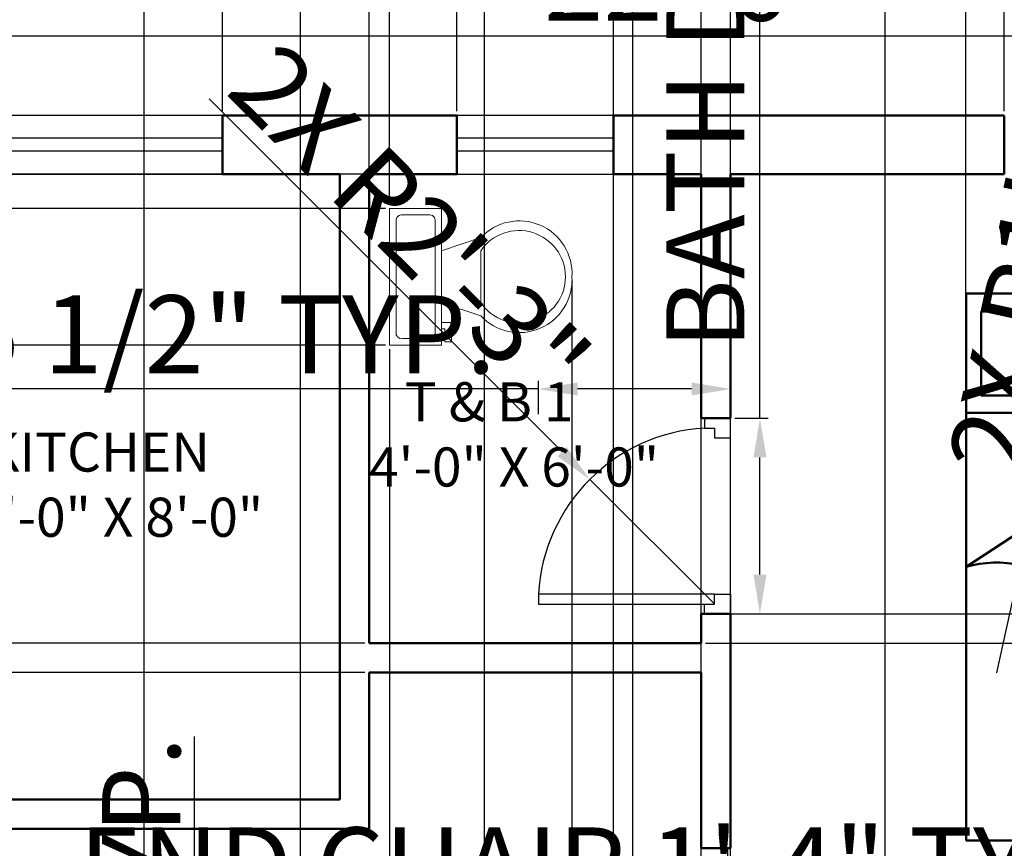
# Model space of a CAD drawing. Units: inches. Extents: x 1086 to 1501, y 383 to 973.
# Tile 5 of 7: x 1165 to 1316, y 723 to 850. Entities that reach past the tile are written whole.
import ezdxf

# ---------------------------------------------------------------- set-up
doc = ezdxf.new("R2010")
doc.units = ezdxf.units.IN
for name, color, linetype, lineweight in [('A-ANNO-DIMS', 2, 'Continuous', 18), ('A-AREA-IDEN', 7, 'Continuous', 25), ('A-FLOR-FIXT', 9, 'Continuous', 18), ('door', 10, 'Continuous', 25), ('furniture', 255, 'Continuous', 18), ('ventilator', 151, 'Continuous', 25), ('wall', 7, 'Continuous', 50), ('window', 81, 'Continuous', 25)]:
    doc.layers.add(name, color=color, linetype=linetype, lineweight=lineweight)
doc.styles.get("Standard").update_dxf_attribs({"font": 'arial.ttf'})
doc.dimstyles.new('ISO-25', dxfattribs={"dimtxt": 12, "dimasz": 6, "dimexe": 1.25, "dimexo": 0.625, "dimtad": 1, "dimdec": 1, "dimlunit": 3, "dimtxsty": 'Standard', "dimcen": 2.5, "dimadec": 0, "dimazin": 0, "dimtfac": 1, "dimtdec": 1, "dimtmove": 0, "dimatfit": 3, "dimfxl": 1, "dimarcsym": 0})

# ---------------------------------------------------------------- blocks, each defined once
blk = doc.blocks.new('w1')
at = {"layer": 'window'}
for p, q in [((1475.33, 845.32), (1475.33, 809.32)), ((1477.33, 845.32), (1477.33, 809.32))]:
    blk.add_line(p, q, dxfattribs=at)
blk.add_lwpolyline([(1471.83, 809.32), (1480.83, 809.32), (1480.83, 845.32), (1471.83, 845.32)], close=True, dxfattribs=at)
blk = doc.blocks.new('v')
at = {"layer": 'ventilator'}
for p, q in [((1539.56, 920.22), (1539.56, 896.22)), ((1541.56, 920.22), (1541.56, 896.22))]:
    blk.add_line(p, q, dxfattribs=at)
blk.add_lwpolyline([(1536.06, 896.22), (1545.06, 896.22), (1545.06, 920.22), (1536.06, 920.22)], close=True, dxfattribs=at)
blk = doc.blocks.new('d2')
at = {"layer": 'door'}
blk.add_line((1603.89, 600.63), (1639.89, 600.63), dxfattribs=at)
blk.add_lwpolyline([(1605.39, 603.13), (1606.89, 603.13), (1606.89, 636.13), (1605.39, 636.13)], close=True, dxfattribs=at)
for points in [[(1606.89, 600.63), (1603.89, 600.63), (1603.89, 604.63), (1605.39, 604.63), (1605.39, 603.13), (1606.89, 603.13), (1606.89, 600.63)], [(1636.89, 600.63), (1639.89, 600.63), (1639.89, 604.63), (1638.39, 604.63), (1638.39, 603.13), (1636.89, 603.13), (1636.89, 600.63)]]:
    blk.add_lwpolyline(points, dxfattribs=at)
blk.add_arc((1605.39, 603.13), 33.03, 2.6026, 87.3974, dxfattribs=at)
blk = doc.blocks.new('d1')
at = {"layer": 'door'}
blk.add_line((1603.89, 536.69), (1633.89, 536.69), dxfattribs=at)
blk.add_lwpolyline([(1605.39, 539.19), (1606.89, 539.19), (1606.89, 566.19), (1605.39, 566.19)], close=True, dxfattribs=at)
for points in [[(1606.89, 536.69), (1603.89, 536.69), (1603.89, 540.69), (1605.39, 540.69), (1605.39, 539.19), (1606.89, 539.19), (1606.89, 536.69)], [(1630.89, 536.69), (1633.89, 536.69), (1633.89, 540.69), (1632.39, 540.69), (1632.39, 539.19), (1630.89, 539.19), (1630.89, 536.69)]]:
    blk.add_lwpolyline(points, dxfattribs=at)
blk.add_arc((1605.39, 539.19), 27.04, 3.1798, 86.8202, dxfattribs=at)
blk = doc.blocks.new('bed')
at = {"layer": 'wall'}
for p, q in [((1549.71, 859.44), (1621.71, 859.44)), ((1585.71, 859.44), (1549.71, 835.76)), ((1585.71, 859.44), (1565.54, 832.3)), ((1585.71, 859.44), (1621.71, 835.76)), ((1585.71, 859.44), (1605.88, 832.3))]:
    blk.add_line(p, q, dxfattribs=at)
for points in [[(1549.71, 793.76), (1621.71, 793.76), (1621.71, 877.76), (1549.71, 877.76)], [(1552.04, 875), (1583.04, 875), (1583.04, 862.08), (1552.04, 862.08)], [(1586.71, 875), (1617.71, 875), (1617.71, 862.08), (1586.71, 862.08)]]:
    blk.add_lwpolyline(points, close=True, dxfattribs=at)
for centre, radius, start, end in [((1554.45, 819.53), 16.91, 49.0428, 106.2967), ((1616.39, 822.13), 14.63, 68.7093, 135.9513)]:
    blk.add_arc(centre, radius, start, end, dxfattribs=at)
blk = doc.blocks.new('*U8')
for p, q in [((241.3, -152.4), (241.3, -50.8)), ((-254, -215.9), (-203.2, -215.9)), ((-254, -241.3), (-254, -215.9)), ((-203.2, -215.9), (-203.2, -203.2)), ((-177.8, -203.2), (-177.8, -241.3)), ((-101.6, -203.2), (-152.4, -355.6)), ((101.6, -203.2), (152.4, -355.6)), ((-177.8, -241.3), (-254, -241.3)), ((101.6, -355.6), (-101.6, -355.6))]:
    blk.add_line(p, q)
blk.add_lwpolyline([(266.7, -203.2), (266.7, 0), (-266.7, 0), (-266.7, -203.2)], close=True)
for points in [[(215.9, -25.4), (-215.9, -25.4)], [(-241.3, -50.8), (-241.3, -152.4)], [(-215.9, -177.8), (215.9, -177.8)]]:
    blk.add_lwpolyline(points)
for centre, radius, start, end in [((-219.075, -47.625), 22.45064, 81.8699, 188.1301), ((219.075, -47.625), 22.45064, 351.8699, 98.1301), ((-219.075, -155.575), 22.45064, 171.869898, 278.1301), ((219.075, -155.575), 22.45064, 261.8699, 8.1301), ((-12.12088, -505.93752), 205.61935, 133.01722, 273.38), ((0.94996, -504.77674), 181.02486, 124.50543, 269.7), ((-0.94742, -504.77674), 181.02486, 270.3, 55.4946), ((12.12342, -505.93752), 205.61935, 266.62, 46.9828)]:
    blk.add_arc(centre, radius, start, end)
blk = doc.blocks.new('*D9')
at = {"layer": 'A-ANNO-DIMS', "color": 0, "lineweight": -2, "transparency": 16777216}
for p, q in [((1133.43, 835.83), (1133.43, 848.67)), ((1403.43, 835.83), (1403.43, 848.67)), ((1139.43, 847.42), (1397.43, 847.42))]:
    blk.add_line(p, q, dxfattribs=at)
at = {"layer": 'A-ANNO-DIMS', "color": 0, "transparency": 16777216}
for points in [[(1139.43, 848.42), (1139.43, 846.42), (1133.43, 847.42)], [(1397.43, 848.42), (1397.43, 846.42), (1403.43, 847.42)]]:
    blk.add_solid(points, dxfattribs=at)
at = {"layer": 'Defpoints', "color": 0, "transparency": 16777216}
for p in [(1403.43, 847.42), (1133.43, 835.21), (1403.43, 835.21)]:
    blk.add_point(p, dxfattribs=at)
at = {"layer": 'A-ANNO-DIMS', "color": 0, "transparency": 16777216, "insert": (1268.43, 854.18), "char_height": 12, "attachment_point": 5}
blk.add_mtext('22\'-6"', dxfattribs=at)
blk = doc.blocks.new('*D17')
at = {"layer": 'A-ANNO-DIMS', "color": 0, "lineweight": -2, "transparency": 16777216}
for p, q in [((1278.93, 788.71), (1278.93, 972.89)), ((1275.05, 788.71), (1280.18, 788.71)), ((1278.93, 764.71), (1278.93, 782.71)), ((1275.05, 758.71), (1280.18, 758.71))]:
    blk.add_line(p, q, dxfattribs=at)
at = {"layer": 'A-ANNO-DIMS', "color": 0, "transparency": 16777216}
for points in [[(1277.93, 782.71), (1279.93, 782.71), (1278.93, 788.71)], [(1277.93, 764.71), (1279.93, 764.71), (1278.93, 758.71)]]:
    blk.add_solid(points, dxfattribs=at)
at = {"layer": 'Defpoints', "color": 0, "transparency": 16777216}
for p in [(1274.43, 788.71), (1278.93, 788.71), (1274.43, 758.71)]:
    blk.add_point(p, dxfattribs=at)
at = {"layer": 'A-ANNO-DIMS', "color": 0, "transparency": 16777216, "insert": (1272.1, 883.8), "char_height": 12, "attachment_point": 5, "rotation": 90}
blk.add_mtext('BATH DOOR 2\'-6" TYP.', dxfattribs=at)
blk = doc.blocks.new('*D18')
at = {"layer": 'A-ANNO-DIMS', "color": 0, "lineweight": -2, "transparency": 16777216}
for p, q in [((1244.93, 789.33), (1244.93, 794.46)), ((1274.43, 789.33), (1274.43, 794.46)), ((1244.93, 793.21), (1136.37, 793.21)), ((1268.43, 793.21), (1250.93, 793.21))]:
    blk.add_line(p, q, dxfattribs=at)
at = {"layer": 'A-ANNO-DIMS', "color": 0, "transparency": 16777216}
for points in [[(1250.93, 794.21), (1250.93, 792.21), (1244.93, 793.21)], [(1268.43, 794.21), (1268.43, 792.21), (1274.43, 793.21)]]:
    blk.add_solid(points, dxfattribs=at)
at = {"layer": 'Defpoints', "color": 0, "transparency": 16777216}
for p in [(1244.93, 793.21), (1244.93, 788.71), (1274.43, 788.71)]:
    blk.add_point(p, dxfattribs=at)
at = {"layer": 'A-ANNO-DIMS', "color": 0, "transparency": 16777216, "insert": (1187.65, 800.04), "char_height": 12, "attachment_point": 5}
blk.add_mtext('2\'-5 1/2" TYP.', dxfattribs=at)
blk = doc.blocks.new('*D25')
at = {"layer": 'A-ANNO-DIMS', "color": 0, "lineweight": -2, "transparency": 16777216}
for p, q in [((1147.7, 709.78), (1147.7, 712.78)), ((1163.51, 709.78), (1163.51, 712.78)), ((1153.7, 711.53), (1157.51, 711.53)), ((1163.51, 711.53), (1340.15, 711.53))]:
    blk.add_line(p, q, dxfattribs=at)
at = {"layer": 'A-ANNO-DIMS', "color": 0, "transparency": 16777216}
for points in [[(1153.7, 712.53), (1153.7, 710.53), (1147.7, 711.53)], [(1157.51, 712.53), (1157.51, 710.53), (1163.51, 711.53)]]:
    blk.add_solid(points, dxfattribs=at)
at = {"layer": 'Defpoints', "color": 0, "transparency": 16777216}
for p in [(1163.51, 711.53), (1147.7, 709.16), (1163.51, 709.16)]:
    blk.add_point(p, dxfattribs=at)
at = {"layer": 'A-ANNO-DIMS', "color": 0, "transparency": 16777216, "insert": (1254.83, 718.36), "char_height": 12, "attachment_point": 5}
blk.add_mtext('END CHAIR 1\'-4" TYP.', dxfattribs=at)
blk = doc.blocks.new('*D28')
at = {"layer": 'A-ANNO-DIMS', "color": 0, "lineweight": -2, "transparency": 16777216}
for p, q in [((1192.17, 660.6), (1192.17, 739.87)), ((1190.08, 660.6), (1193.42, 660.6)), ((1192.17, 650.79), (1192.17, 654.6)), ((1190.08, 644.79), (1193.42, 644.79))]:
    blk.add_line(p, q, dxfattribs=at)
at = {"layer": 'A-ANNO-DIMS', "color": 0, "transparency": 16777216}
for points in [[(1191.17, 654.6), (1193.17, 654.6), (1192.17, 660.6)], [(1191.17, 650.79), (1193.17, 650.79), (1192.17, 644.79)]]:
    blk.add_solid(points, dxfattribs=at)
at = {"layer": 'Defpoints', "color": 0, "transparency": 16777216}
for p in [(1189.45, 660.6), (1192.17, 660.6), (1189.45, 644.79)]:
    blk.add_point(p, dxfattribs=at)
at = {"layer": 'A-ANNO-DIMS', "color": 0, "transparency": 16777216, "insert": (1185.52, 703.24), "char_height": 12, "attachment_point": 5, "rotation": 90}
blk.add_mtext('1\'-4" TYP.', dxfattribs=at)
blk = doc.blocks.new('*D29')
at = {"layer": 'A-ANNO-DIMS', "color": 0, "lineweight": -2, "transparency": 16777216}
for p, q in [((1133.43, 835.83), (1133.43, 867.19)), ((1139.43, 865.94), (1154.43, 865.94)), ((1160.43, 835.83), (1160.43, 867.19)), ((1160.43, 865.94), (1199.78, 865.94))]:
    blk.add_line(p, q, dxfattribs=at)
at = {"layer": 'A-ANNO-DIMS', "color": 0, "transparency": 16777216}
for points in [[(1139.43, 866.94), (1139.43, 864.94), (1133.43, 865.94)], [(1154.43, 866.94), (1154.43, 864.94), (1160.43, 865.94)]]:
    blk.add_solid(points, dxfattribs=at)
at = {"layer": 'Defpoints', "color": 0, "transparency": 16777216}
for p in [(1160.43, 865.94), (1133.43, 835.21), (1160.43, 835.21)]:
    blk.add_point(p, dxfattribs=at)
at = {"layer": 'A-ANNO-DIMS', "color": 0, "transparency": 16777216, "insert": (1183.11, 872.7), "char_height": 12, "attachment_point": 5}
blk.add_mtext('2\'-3"', dxfattribs=at)
blk = doc.blocks.new('*D30')
at = {"layer": 'A-ANNO-DIMS', "color": 0, "lineweight": -2, "transparency": 16777216}
for p, q in [((1196.43, 835.83), (1196.43, 867.19)), ((1202.43, 865.94), (1226.43, 865.94)), ((1232.43, 835.83), (1232.43, 867.19))]:
    blk.add_line(p, q, dxfattribs=at)
at = {"layer": 'A-ANNO-DIMS', "color": 0, "transparency": 16777216}
for points in [[(1202.43, 866.94), (1202.43, 864.94), (1196.43, 865.94)], [(1226.43, 866.94), (1226.43, 864.94), (1232.43, 865.94)]]:
    blk.add_solid(points, dxfattribs=at)
at = {"layer": 'Defpoints', "color": 0, "transparency": 16777216}
for p in [(1232.43, 865.94), (1196.43, 835.21), (1232.43, 835.21)]:
    blk.add_point(p, dxfattribs=at)
at = {"layer": 'A-ANNO-DIMS', "color": 0, "transparency": 16777216, "insert": (1214.43, 872.7), "char_height": 12, "attachment_point": 5}
blk.add_mtext('3\'-0"', dxfattribs=at)
blk = doc.blocks.new('*D31')
at = {"layer": 'A-ANNO-DIMS', "color": 0, "lineweight": -2, "transparency": 16777216}
for p, q in [((1256.43, 835.83), (1256.43, 867.19)), ((1262.43, 865.94), (1310.43, 865.94)), ((1316.43, 835.83), (1316.43, 867.19))]:
    blk.add_line(p, q, dxfattribs=at)
at = {"layer": 'A-ANNO-DIMS', "color": 0, "transparency": 16777216}
for points in [[(1262.43, 866.94), (1262.43, 864.94), (1256.43, 865.94)], [(1310.43, 866.94), (1310.43, 864.94), (1316.43, 865.94)]]:
    blk.add_solid(points, dxfattribs=at)
at = {"layer": 'Defpoints', "color": 0, "transparency": 16777216}
for p in [(1316.43, 865.94), (1256.43, 835.21), (1316.43, 835.21)]:
    blk.add_point(p, dxfattribs=at)
at = {"layer": 'A-ANNO-DIMS', "color": 0, "transparency": 16777216, "insert": (1286.43, 872.69), "char_height": 12, "attachment_point": 5}
blk.add_mtext('5\'-0"', dxfattribs=at)
blk = doc.blocks.new('*D40')
at = {"layer": 'A-ANNO-DIMS', "color": 0, "lineweight": -2, "transparency": 16777216}
for p, q in [((1142.43, 502.33), (1142.43, 867.19)), ((1148.43, 865.94), (1263.93, 865.94)), ((1269.93, 502.33), (1269.93, 867.19))]:
    blk.add_line(p, q, dxfattribs=at)
at = {"layer": 'A-ANNO-DIMS', "color": 0, "transparency": 16777216}
for points in [[(1148.43, 866.94), (1148.43, 864.94), (1142.43, 865.94)], [(1263.93, 866.94), (1263.93, 864.94), (1269.93, 865.94)]]:
    blk.add_solid(points, dxfattribs=at)
at = {"layer": 'Defpoints', "color": 0, "transparency": 16777216}
for p in [(1269.93, 865.94), (1142.43, 501.71), (1269.93, 501.71)]:
    blk.add_point(p, dxfattribs=at)
at = {"layer": 'A-ANNO-DIMS', "color": 0, "transparency": 16777216, "insert": (1206.18, 872.77), "char_height": 12, "attachment_point": 5}
blk.add_mtext('10\'-7 1/2"', dxfattribs=at)
blk = doc.blocks.new('*D42')
at = {"layer": 'A-ANNO-DIMS', "color": 0, "lineweight": -2, "transparency": 16777216}
for p, q in [((1256.43, 502.33), (1256.43, 867.19)), ((1262.43, 865.94), (1263.93, 865.94)), ((1269.93, 502.33), (1269.93, 867.19)), ((1269.93, 865.94), (1335.91, 865.94))]:
    blk.add_line(p, q, dxfattribs=at)
at = {"layer": 'A-ANNO-DIMS', "color": 0, "transparency": 16777216}
for points in [[(1262.43, 866.94), (1262.43, 864.94), (1256.43, 865.94)], [(1263.93, 866.94), (1263.93, 864.94), (1269.93, 865.94)]]:
    blk.add_solid(points, dxfattribs=at)
at = {"layer": 'Defpoints', "color": 0, "transparency": 16777216}
for p in [(1269.93, 865.94), (1256.43, 501.71), (1269.93, 501.71)]:
    blk.add_point(p, dxfattribs=at)
at = {"layer": 'A-ANNO-DIMS', "color": 0, "transparency": 16777216, "insert": (1305.92, 872.77), "char_height": 12, "attachment_point": 5}
blk.add_mtext('1\'-1 1/2"', dxfattribs=at)
blk = doc.blocks.new('*D43')
at = {"layer": 'A-ANNO-DIMS', "color": 0, "lineweight": -2, "transparency": 16777216}
for p, q in [((1208.43, 497.83), (1208.43, 867.19)), ((1214.43, 865.94), (1250.43, 865.94)), ((1256.43, 497.83), (1256.43, 867.19))]:
    blk.add_line(p, q, dxfattribs=at)
at = {"layer": 'A-ANNO-DIMS', "color": 0, "transparency": 16777216}
for points in [[(1214.43, 866.94), (1214.43, 864.94), (1208.43, 865.94)], [(1250.43, 866.94), (1250.43, 864.94), (1256.43, 865.94)]]:
    blk.add_solid(points, dxfattribs=at)
at = {"layer": 'Defpoints', "color": 0, "transparency": 16777216}
for p in [(1256.43, 865.94), (1208.43, 497.21), (1256.43, 497.21)]:
    blk.add_point(p, dxfattribs=at)
at = {"layer": 'A-ANNO-DIMS', "color": 0, "transparency": 16777216, "insert": (1232.43, 872.69), "char_height": 12, "attachment_point": 5}
blk.add_mtext('4\'-0"', dxfattribs=at)
blk = doc.blocks.new('*D45')
at = {"layer": 'A-ANNO-DIMS', "color": 0, "lineweight": -2, "transparency": 16777216}
for p, q in [((1259.43, 497.83), (1259.43, 867.19)), ((1265.43, 865.94), (1352.43, 865.94)), ((1358.43, 497.83), (1358.43, 867.19))]:
    blk.add_line(p, q, dxfattribs=at)
at = {"layer": 'A-ANNO-DIMS', "color": 0, "transparency": 16777216}
for points in [[(1265.43, 866.94), (1265.43, 864.94), (1259.43, 865.94)], [(1352.43, 866.94), (1352.43, 864.94), (1358.43, 865.94)]]:
    blk.add_solid(points, dxfattribs=at)
at = {"layer": 'Defpoints', "color": 0, "transparency": 16777216}
for p in [(1358.43, 865.94), (1259.43, 497.21), (1358.43, 497.21)]:
    blk.add_point(p, dxfattribs=at)
at = {"layer": 'A-ANNO-DIMS', "color": 0, "transparency": 16777216, "insert": (1308.93, 872.7), "char_height": 12, "attachment_point": 5}
blk.add_mtext('8\'-3"', dxfattribs=at)
blk = doc.blocks.new('*D49')
at = {"layer": 'A-ANNO-DIMS', "color": 0, "lineweight": -2, "transparency": 16777216}
for p, q in [((1110.93, 760.21), (1110.93, 766.21)), ((1218.3, 754.21), (1109.68, 754.21)), ((1110.93, 754.21), (1110.93, 749.71)), ((1218.3, 749.71), (1109.68, 749.71)), ((1110.93, 743.71), (1110.93, 676.6))]:
    blk.add_line(p, q, dxfattribs=at)
at = {"layer": 'A-ANNO-DIMS', "color": 0, "transparency": 16777216}
for points in [[(1109.93, 760.21), (1111.93, 760.21), (1110.93, 754.21)], [(1109.93, 743.71), (1111.93, 743.71), (1110.93, 749.71)]]:
    blk.add_solid(points, dxfattribs=at)
at = {"layer": 'Defpoints', "color": 0, "transparency": 16777216}
for p in [(1218.93, 754.21), (1110.93, 749.71), (1218.93, 749.71)]:
    blk.add_point(p, dxfattribs=at)
at = {"layer": 'A-ANNO-DIMS', "color": 0, "transparency": 16777216, "insert": (1104.1, 707.15), "char_height": 12, "attachment_point": 5, "rotation": 90}
blk.add_mtext('0\'-4 1/2"', dxfattribs=at)
blk = doc.blocks.new('*D50')
at = {"layer": 'A-ANNO-DIMS', "color": 0, "lineweight": -2, "transparency": 16777216}
for p, q in [((1184.43, 502.33), (1184.43, 867.19)), ((1190.43, 865.94), (1202.43, 865.94)), ((1208.43, 502.33), (1208.43, 867.19)), ((1208.43, 865.94), (1247.78, 865.94))]:
    blk.add_line(p, q, dxfattribs=at)
at = {"layer": 'A-ANNO-DIMS', "color": 0, "transparency": 16777216}
for points in [[(1190.43, 866.94), (1190.43, 864.94), (1184.43, 865.94)], [(1202.43, 866.94), (1202.43, 864.94), (1208.43, 865.94)]]:
    blk.add_solid(points, dxfattribs=at)
at = {"layer": 'Defpoints', "color": 0, "transparency": 16777216}
for p in [(1208.43, 865.94), (1184.43, 501.71), (1208.43, 501.71)]:
    blk.add_point(p, dxfattribs=at)
at = {"layer": 'A-ANNO-DIMS', "color": 0, "transparency": 16777216, "insert": (1231.11, 872.69), "char_height": 12, "attachment_point": 5}
blk.add_mtext('2\'-0"', dxfattribs=at)
blk = doc.blocks.new('*D52')
at = {"layer": 'A-ANNO-DIMS', "color": 0, "lineweight": -2, "transparency": 16777216}
for p, q in [((1110.93, 692.71), (1110.93, 759.82)), ((1273.8, 686.71), (1109.68, 686.71)), ((1110.93, 682.21), (1110.93, 686.71)), ((1273.8, 682.21), (1109.68, 682.21)), ((1110.93, 676.21), (1110.93, 670.21))]:
    blk.add_line(p, q, dxfattribs=at)
at = {"layer": 'A-ANNO-DIMS', "color": 0, "transparency": 16777216}
for points in [[(1109.93, 692.71), (1111.93, 692.71), (1110.93, 686.71)], [(1109.93, 676.21), (1111.93, 676.21), (1110.93, 682.21)]]:
    blk.add_solid(points, dxfattribs=at)
at = {"layer": 'Defpoints', "color": 0, "transparency": 16777216}
for p in [(1110.93, 686.71), (1274.43, 686.71), (1274.43, 682.21)]:
    blk.add_point(p, dxfattribs=at)
at = {"layer": 'A-ANNO-DIMS', "color": 0, "transparency": 16777216, "insert": (1104.1, 729.26), "char_height": 12, "attachment_point": 5, "rotation": 90}
blk.add_mtext('0\'-4 1/2"', dxfattribs=at)
blk = doc.blocks.new('*D53')
at = {"layer": 'A-ANNO-DIMS', "color": 0, "lineweight": -2, "transparency": 16777216}
for p, q in [((1110.93, 686.71), (1110.93, 752.69)), ((1269.3, 686.71), (1109.68, 686.71)), ((1110.93, 679.21), (1110.93, 680.71)), ((1269.3, 673.21), (1109.68, 673.21))]:
    blk.add_line(p, q, dxfattribs=at)
at = {"layer": 'A-ANNO-DIMS', "color": 0, "transparency": 16777216}
for points in [[(1109.93, 680.71), (1111.93, 680.71), (1110.93, 686.71)], [(1109.93, 679.21), (1111.93, 679.21), (1110.93, 673.21)]]:
    blk.add_solid(points, dxfattribs=at)
at = {"layer": 'Defpoints', "color": 0, "transparency": 16777216}
for p in [(1110.93, 686.71), (1269.93, 686.71), (1269.93, 673.21)]:
    blk.add_point(p, dxfattribs=at)
at = {"layer": 'A-ANNO-DIMS', "color": 0, "transparency": 16777216, "insert": (1104.1, 722.7), "char_height": 12, "attachment_point": 5, "rotation": 90}
blk.add_mtext('1\'-1 1/2"', dxfattribs=at)
blk = doc.blocks.new('*D54')
at = {"layer": 'A-ANNO-DIMS', "color": 0, "lineweight": -2, "transparency": 16777216}
for p, q in [((1427.11, 764.71), (1427.11, 831.82)), ((1270.55, 758.71), (1428.36, 758.71)), ((1427.11, 754.21), (1427.11, 758.71)), ((1270.55, 754.21), (1428.36, 754.21)), ((1427.11, 748.21), (1427.11, 742.21))]:
    blk.add_line(p, q, dxfattribs=at)
at = {"layer": 'A-ANNO-DIMS', "color": 0, "transparency": 16777216}
for points in [[(1426.11, 764.71), (1428.11, 764.71), (1427.11, 758.71)], [(1426.11, 748.21), (1428.11, 748.21), (1427.11, 754.21)]]:
    blk.add_solid(points, dxfattribs=at)
at = {"layer": 'Defpoints', "color": 0, "transparency": 16777216}
for p in [(1269.93, 758.71), (1427.11, 758.71), (1269.93, 754.21)]:
    blk.add_point(p, dxfattribs=at)
at = {"layer": 'A-ANNO-DIMS', "color": 0, "transparency": 16777216, "insert": (1420.28, 801.26), "char_height": 12, "attachment_point": 5, "rotation": 90}
blk.add_mtext('0\'-4 1/2"', dxfattribs=at)
blk = doc.blocks.new('*D55')
at = {"layer": 'A-ANNO-DIMS', "color": 0, "lineweight": -2, "transparency": 16777216}
for p, q in [((1212.93, 865.94), (1206.93, 865.94)), ((1218.93, 826.83), (1218.93, 867.19)), ((1218.93, 865.94), (1222.08, 865.94)), ((1222.08, 821.57), (1222.08, 867.19)), ((1228.08, 865.94), (1267.23, 865.94))]:
    blk.add_line(p, q, dxfattribs=at)
at = {"layer": 'A-ANNO-DIMS', "color": 0, "transparency": 16777216}
for points in [[(1212.93, 866.94), (1212.93, 864.94), (1218.93, 865.94)], [(1228.08, 866.94), (1228.08, 864.94), (1222.08, 865.94)]]:
    blk.add_solid(points, dxfattribs=at)
at = {"layer": 'Defpoints', "color": 0, "transparency": 16777216}
for p in [(1222.08, 865.94), (1218.93, 826.21), (1222.08, 820.94)]:
    blk.add_point(p, dxfattribs=at)
at = {"layer": 'A-ANNO-DIMS', "color": 0, "transparency": 16777216, "insert": (1250.66, 872.7), "char_height": 12, "attachment_point": 5}
blk.add_mtext('0\'-3"', dxfattribs=at)
blk = doc.blocks.new('*D56')
at = {"layer": 'A-ANNO-DIMS', "color": 0, "lineweight": -2, "transparency": 16777216}
for p, q in [((1110.93, 832.21), (1110.93, 838.21)), ((1218.3, 826.21), (1109.68, 826.21)), ((1110.93, 826.21), (1110.93, 820.94)), ((1221.46, 820.94), (1109.68, 820.94)), ((1110.93, 814.94), (1110.93, 747.83))]:
    blk.add_line(p, q, dxfattribs=at)
at = {"layer": 'A-ANNO-DIMS', "color": 0, "transparency": 16777216}
for points in [[(1109.93, 832.21), (1111.93, 832.21), (1110.93, 826.21)], [(1109.93, 814.94), (1111.93, 814.94), (1110.93, 820.94)]]:
    blk.add_solid(points, dxfattribs=at)
at = {"layer": 'Defpoints', "color": 0, "transparency": 16777216}
for p in [(1218.93, 826.21), (1110.93, 820.94), (1222.08, 820.94)]:
    blk.add_point(p, dxfattribs=at)
at = {"layer": 'A-ANNO-DIMS', "color": 0, "transparency": 16777216, "insert": (1104.1, 778.39), "char_height": 12, "attachment_point": 5, "rotation": 90}
blk.add_mtext('0\'-5 1/2"', dxfattribs=at)
blk = doc.blocks.new('*D57')
at = {"layer": 'A-ANNO-DIMS', "color": 0, "lineweight": -2, "transparency": 16777216}
for p, q in [((1110.93, 820.94), (1110.93, 858.96)), ((1221.46, 820.94), (1109.68, 820.94)), ((1110.93, 805.94), (1110.93, 814.94)), ((1221.46, 799.94), (1109.68, 799.94))]:
    blk.add_line(p, q, dxfattribs=at)
at = {"layer": 'A-ANNO-DIMS', "color": 0, "transparency": 16777216}
for points in [[(1109.93, 814.94), (1111.93, 814.94), (1110.93, 820.94)], [(1109.93, 805.94), (1111.93, 805.94), (1110.93, 799.94)]]:
    blk.add_solid(points, dxfattribs=at)
at = {"layer": 'Defpoints', "color": 0, "transparency": 16777216}
for p in [(1110.93, 820.94), (1222.08, 820.94), (1222.08, 799.94)]:
    blk.add_point(p, dxfattribs=at)
at = {"layer": 'A-ANNO-DIMS', "color": 0, "transparency": 16777216, "insert": (1104.18, 842.95), "char_height": 12, "attachment_point": 5, "rotation": 90}
blk.add_mtext('1\'-9"', dxfattribs=at)
blk = doc.blocks.new('*D58')
at = {"layer": 'A-ANNO-DIMS', "color": 0, "lineweight": -2, "transparency": 16777216}
for p, q in [((1250.08, 809.82), (1250.08, 392.46)), ((1222.08, 799.32), (1222.08, 392.46)), ((1228.08, 393.71), (1244.08, 393.71)), ((1250.08, 393.71), (1289.44, 393.71))]:
    blk.add_line(p, q, dxfattribs=at)
at = {"layer": 'A-ANNO-DIMS', "color": 0, "transparency": 16777216}
for points in [[(1228.08, 394.71), (1228.08, 392.71), (1222.08, 393.71)], [(1244.08, 394.71), (1244.08, 392.71), (1250.08, 393.71)]]:
    blk.add_solid(points, dxfattribs=at)
at = {"layer": 'Defpoints', "color": 0, "transparency": 16777216}
for p in [(1250.08, 810.44), (1222.08, 799.94), (1250.08, 393.71)]:
    blk.add_point(p, dxfattribs=at)
at = {"layer": 'A-ANNO-DIMS', "color": 0, "transparency": 16777216, "insert": (1272.76, 400.36), "char_height": 12, "attachment_point": 5}
blk.add_mtext('2\'-4"', dxfattribs=at)
blk = doc.blocks.new('*D59')
at = {"layer": 'A-ANNO-DIMS', "color": 0, "lineweight": -2, "transparency": 16777216}
for p, q in [((1218.93, 826.83), (1218.93, 867.19)), ((1224.93, 865.94), (1263.93, 865.94)), ((1269.93, 826.83), (1269.93, 867.19))]:
    blk.add_line(p, q, dxfattribs=at)
at = {"layer": 'A-ANNO-DIMS', "color": 0, "transparency": 16777216}
for points in [[(1224.93, 866.94), (1224.93, 864.94), (1218.93, 865.94)], [(1263.93, 866.94), (1263.93, 864.94), (1269.93, 865.94)]]:
    blk.add_solid(points, dxfattribs=at)
at = {"layer": 'Defpoints', "color": 0, "transparency": 16777216}
for p in [(1269.93, 865.94), (1218.93, 826.21), (1269.93, 826.21)]:
    blk.add_point(p, dxfattribs=at)
at = {"layer": 'A-ANNO-DIMS', "color": 0, "transparency": 16777216, "insert": (1244.43, 872.7), "char_height": 12, "attachment_point": 5}
blk.add_mtext('4\'-3"', dxfattribs=at)
blk = doc.blocks.new('*D61')
at = {"layer": 'A-ANNO-DIMS', "color": 0, "lineweight": -2, "transparency": 16777216}
for p, q in [((1376.11, 865.94), (1310.13, 865.94)), ((1382.11, 674.69), (1382.11, 867.19)), ((1394.43, 865.94), (1382.11, 865.94)), ((1394.43, 678.33), (1394.43, 867.19)), ((1400.43, 865.94), (1406.43, 865.94))]:
    blk.add_line(p, q, dxfattribs=at)
at = {"layer": 'A-ANNO-DIMS', "color": 0, "transparency": 16777216}
for points in [[(1376.11, 866.94), (1376.11, 864.94), (1382.11, 865.94)], [(1400.43, 866.94), (1400.43, 864.94), (1394.43, 865.94)]]:
    blk.add_solid(points, dxfattribs=at)
at = {"layer": 'Defpoints', "color": 0, "transparency": 16777216}
for p in [(1382.11, 865.94), (1394.43, 677.71), (1382.11, 674.06)]:
    blk.add_point(p, dxfattribs=at)
at = {"layer": 'A-ANNO-DIMS', "color": 0, "transparency": 16777216, "insert": (1340.12, 872.77), "char_height": 12, "attachment_point": 5}
blk.add_mtext('1\'-0 1/2"', dxfattribs=at)
blk = doc.blocks.new('*D69')
at = {"layer": 'A-ANNO-DIMS', "color": 0, "lineweight": -2, "transparency": 16777216}
for p, q in [((1236.63, 603.21), (1236.63, 867.19)), ((1242.63, 865.94), (1263.93, 865.94)), ((1269.93, 603.25), (1269.93, 867.19)), ((1269.93, 865.94), (1337.25, 865.94))]:
    blk.add_line(p, q, dxfattribs=at)
at = {"layer": 'A-ANNO-DIMS', "color": 0, "transparency": 16777216}
for points in [[(1242.63, 866.94), (1242.63, 864.94), (1236.63, 865.94)], [(1263.93, 866.94), (1263.93, 864.94), (1269.93, 865.94)]]:
    blk.add_solid(points, dxfattribs=at)
at = {"layer": 'Defpoints', "color": 0, "transparency": 16777216}
for p in [(1269.93, 865.94), (1236.63, 602.59), (1269.93, 602.62)]:
    blk.add_point(p, dxfattribs=at)
at = {"layer": 'A-ANNO-DIMS', "color": 0, "transparency": 16777216, "insert": (1306.59, 872.77), "char_height": 12, "attachment_point": 5}
blk.add_mtext('2\'-9 1/2"', dxfattribs=at)
blk = doc.blocks.new('*D71')
at = {"layer": 'A-ANNO-DIMS', "color": 0, "lineweight": -2, "transparency": 16777216}
for p, q in [((1142.43, 589.29), (1142.43, 867.19)), ((1148.43, 865.94), (1154.43, 865.94)), ((1160.43, 589.29), (1160.43, 867.19)), ((1160.43, 865.94), (1198.45, 865.94))]:
    blk.add_line(p, q, dxfattribs=at)
at = {"layer": 'A-ANNO-DIMS', "color": 0, "transparency": 16777216}
for points in [[(1148.43, 866.94), (1148.43, 864.94), (1142.43, 865.94)], [(1154.43, 866.94), (1154.43, 864.94), (1160.43, 865.94)]]:
    blk.add_solid(points, dxfattribs=at)
at = {"layer": 'Defpoints', "color": 0, "transparency": 16777216}
for p in [(1160.43, 865.94), (1142.43, 588.67), (1160.43, 588.67)]:
    blk.add_point(p, dxfattribs=at)
at = {"layer": 'A-ANNO-DIMS', "color": 0, "transparency": 16777216, "insert": (1182.44, 872.69), "char_height": 12, "attachment_point": 5}
blk.add_mtext('1\'-6"', dxfattribs=at)
blk = doc.blocks.new('*D75')
at = {"layer": 'A-ANNO-DIMS', "color": 0, "lineweight": -2, "transparency": 16777216}
for p, q in [((1274.43, 723.33), (1274.43, 867.19)), ((1280.43, 865.94), (1304.55, 865.94)), ((1310.55, 724.51), (1310.55, 867.19))]:
    blk.add_line(p, q, dxfattribs=at)
at = {"layer": 'A-ANNO-DIMS', "color": 0, "transparency": 16777216}
for points in [[(1280.43, 866.94), (1280.43, 864.94), (1274.43, 865.94)], [(1304.55, 866.94), (1304.55, 864.94), (1310.55, 865.94)]]:
    blk.add_solid(points, dxfattribs=at)
at = {"layer": 'Defpoints', "color": 0, "transparency": 16777216}
for p in [(1310.55, 865.94), (1310.55, 723.89), (1274.43, 722.71)]:
    blk.add_point(p, dxfattribs=at)
at = {"layer": 'A-ANNO-DIMS', "color": 0, "transparency": 16777216, "insert": (1292.49, 872.7), "char_height": 12, "attachment_point": 5}
blk.add_mtext('3\'-0"', dxfattribs=at)
blk = doc.blocks.new('*D77')
at = {"layer": 'A-ANNO-DIMS', "color": 0, "lineweight": -2, "transparency": 16777216}
for p, q in [((1274.43, 502.33), (1274.43, 867.19)), ((1280.43, 865.94), (1292.14, 865.94)), ((1298.14, 513.04), (1298.14, 867.19)), ((1298.14, 865.94), (1373.44, 865.94))]:
    blk.add_line(p, q, dxfattribs=at)
at = {"layer": 'A-ANNO-DIMS', "color": 0, "transparency": 16777216}
for points in [[(1280.43, 866.94), (1280.43, 864.94), (1274.43, 865.94)], [(1292.14, 866.94), (1292.14, 864.94), (1298.14, 865.94)]]:
    blk.add_solid(points, dxfattribs=at)
at = {"layer": 'Defpoints', "color": 0, "transparency": 16777216}
for p in [(1298.14, 865.94), (1298.14, 512.42), (1274.43, 501.71)]:
    blk.add_point(p, dxfattribs=at)
at = {"layer": 'A-ANNO-DIMS', "color": 0, "transparency": 16777216, "insert": (1338.79, 872.77), "char_height": 12, "attachment_point": 5}
blk.add_mtext('1\'-11 1/2"', dxfattribs=at)
blk = doc.blocks.new('*D79')
at = {"layer": 'A-ANNO-DIMS', "color": 0, "lineweight": -2, "transparency": 16777216}
for p, q in [((1194.38, 837.75), (1248.57, 783.57)), ((1271.93, 760.21), (1252.81, 779.33))]:
    blk.add_line(p, q, dxfattribs=at)
at = {"layer": 'A-ANNO-DIMS', "color": 0, "transparency": 16777216}
blk.add_solid([(1249.27, 784.28), (1247.86, 782.86), (1252.81, 779.33)], dxfattribs=at)
at = {"layer": 'Defpoints', "color": 0, "transparency": 16777216}
for p in [(1252.81, 779.33), (1271.93, 760.21)]:
    blk.add_point(p, dxfattribs=at)
at = {"layer": 'A-ANNO-DIMS', "color": 0, "transparency": 16777216, "insert": (1224.13, 817.56), "char_height": 12, "attachment_point": 5, "rotation": 315.0007}
blk.add_mtext('2X R2\'-3"', dxfattribs=at)
blk = doc.blocks.new('*D81')
at = {"layer": 'A-ANNO-DIMS', "color": 0, "lineweight": -2, "transparency": 16777216}
for p, q in [((1336.56, 846.9), (1320.19, 772.04)), ((1315.3, 749.66), (1318.91, 766.18))]:
    blk.add_line(p, q, dxfattribs=at)
at = {"layer": 'A-ANNO-DIMS', "color": 0, "transparency": 16777216}
blk.add_solid([(1319.22, 772.25), (1321.17, 771.83), (1318.91, 766.18)], dxfattribs=at)
at = {"layer": 'Defpoints', "color": 0, "transparency": 16777216}
for p in [(1318.91, 766.18), (1315.3, 749.66)]:
    blk.add_point(p, dxfattribs=at)
at = {"layer": 'A-ANNO-DIMS', "color": 0, "transparency": 16777216, "insert": (1322.42, 813.84), "char_height": 12, "attachment_point": 5, "rotation": 77.6694}
blk.add_mtext('2X R1\'-5"', dxfattribs=at)

msp = doc.modelspace()

# ---------------------------------------------------------------- linework, layer by layer
at = {"layer": 'wall'}
for p, q in [((1196.43, 826.21), (1196.43, 835.21)), ((1232.43, 835.21), (1196.43, 835.21)), ((1232.43, 826.21), (1232.43, 835.21)), ((1256.43, 826.21), (1256.43, 835.21)), ((1316.43, 835.21), (1256.43, 835.21)), ((1316.43, 826.21), (1316.43, 835.21)), ((1214.43, 826.21), (1196.43, 826.21)), ((1214.43, 826.21), (1214.43, 730.21)), ((1218.93, 826.21), (1218.93, 754.21)), ((1232.43, 826.21), (1218.93, 826.21)), ((1269.93, 826.21), (1256.43, 826.21)), ((1269.93, 788.71), (1269.93, 826.21)), ((1316.43, 826.21), (1274.43, 826.21)), ((1274.43, 788.71), (1274.43, 826.21)), ((1274.43, 788.71), (1269.93, 788.71)), ((1269.93, 754.21), (1269.93, 758.71)), ((1274.43, 758.71), (1269.93, 758.71)), ((1274.43, 722.71), (1274.43, 758.71)), ((1269.93, 754.21), (1218.93, 754.21)), ((1269.93, 749.71), (1218.93, 749.71)), ((1218.93, 749.71), (1218.93, 725.71)), ((1269.93, 722.71), (1269.93, 749.71)), ((1214.43, 730.21), (1142.43, 730.21)), ((1218.93, 725.71), (1142.43, 725.71)), ((1274.43, 722.71), (1269.93, 722.71))]:
    msp.add_line(p, q, dxfattribs=at)

# ---------------------------------------------------------------- block references
at = {"layer": 'A-FLOR-FIXT', "xscale": 0.0393700787401575, "yscale": 0.0393700787401575, "zscale": 0.0393700787401575, "rotation": 90}
msp.add_blockref('*U8', (1222.08, 810.44), dxfattribs=at)
at = {"layer": 'door', "rotation": 90}
msp.add_blockref('d1', (1811.12, -845.19), dxfattribs=at)
at = {"layer": 'door', "xscale": -1, "rotation": 270}
msp.add_blockref('d2', (669.3, -917.19), dxfattribs=at)
at = {"layer": 'furniture'}
msp.add_blockref('bed', (-239.15, -69.87), dxfattribs=at)
at = {"layer": 'ventilator', "rotation": 270}
msp.add_blockref('v', (336.21, 2371.26), dxfattribs=at)
at = {"layer": 'window', "rotation": 270}
msp.add_blockref('w1', (351.11, 2307.04), dxfattribs=at)

# ---------------------------------------------------------------- texts
at = {"layer": 'A-AREA-IDEN', "char_height": 6, "attachment_point": 1}
for s, insert in [('   T & B 1\\P4\'-0" X 6\'-0"', (1218.93, 794.24)), (' KITCHEN\\P6\'-0" X 8\'-0"', (1158.17, 786.53))]:
    msp.add_mtext_dynamic_manual_height_columns(s, width=53.2651, gutter_width=12.5, heights=[0], dxfattribs=dict(at, insert=insert))

# ---------------------------------------------------------------- dimensions: what is measured, and where the dimension line sits
at = {"layer": 'A-ANNO-DIMS'}
for base, p1, p2, angle, text, picture, middle in [((1278.93, 788.71), (1274.43, 758.71), (1274.43, 788.71), 90, 'BATH DOOR <> TYP.', '*D17', (1272.1, 883.8)), ((1244.93, 793.21), (1274.43, 788.71), (1244.93, 788.71), 180, '<> TYP.', '*D18', (1187.65, 800.04)), ((1192.17, 660.6), (1189.45, 644.79), (1189.45, 660.6), 90, '<> TYP.', '*D28', (1185.52, 703.24))]:
    dim = msp.add_linear_dim(base=base, p1=p1, p2=p2, angle=angle, text=text, dimstyle='ISO-25', override={"dimdec": 1, "dimlfac": 1, "dimrnd": 0, "dimzin": 1, "dimdsep": 46, "dimlunit": 4, "dimfrac": 2}, dxfattribs=at)
    dim.commit()
    dim.dimension.update_dxf_attribs({"geometry": picture, "text_midpoint": middle})
for base, p1, p2, override, picture, middle in [((1269.93, 865.94), (1142.43, 501.71), (1269.93, 501.71), {"dimdec": 1, "dimlfac": 1, "dimrnd": 0, "dimzin": 1, "dimdsep": 46, "dimlunit": 4, "dimfrac": 2}, '*D40', (1206.18, 872.77)), ((1269.93, 865.94), (1236.63, 602.59), (1269.93, 602.62), {"dimdec": 1, "dimlfac": 1, "dimrnd": 0, "dimzin": 1, "dimdsep": 46, "dimlunit": 4, "dimfrac": 2}, '*D69', (1306.59, 872.77)), ((1269.93, 865.94), (1256.43, 501.71), (1269.93, 501.71), {"dimdec": 1, "dimlfac": 1, "dimrnd": 0, "dimzin": 1, "dimdsep": 46, "dimlunit": 4, "dimfrac": 2}, '*D42', (1305.92, 872.77)), ((1298.14, 865.94), (1274.43, 501.71), (1298.14, 512.42), {"dimdec": 1, "dimlfac": 1, "dimrnd": 0, "dimzin": 1, "dimdsep": 46, "dimlunit": 4, "dimfrac": 2}, '*D77', (1338.79, 872.77)), ((1382.11, 865.94), (1394.43, 677.71), (1382.11, 674.06), {"dimdec": 1, "dimlfac": 1, "dimrnd": 0, "dimzin": 1, "dimdsep": 46, "dimlunit": 4, "dimfrac": 2}, '*D61', (1340.12, 872.77)), ((1160.43, 865.94), (1133.43, 835.21), (1160.43, 835.21), {"dimdec": 1, "dimlfac": 1, "dimrnd": 0, "dimzin": 1, "dimdsep": 46, "dimlunit": 4, "dimfrac": 2}, '*D29', (1183.11, 872.7)), ((1160.43, 865.94), (1142.43, 588.67), (1160.43, 588.67), {"dimdec": 1, "dimlfac": 1, "dimrnd": 0, "dimzin": 1, "dimdsep": 46, "dimlunit": 4, "dimfrac": 2}, '*D71', (1182.44, 872.69)), ((1208.43, 865.94), (1184.43, 501.71), (1208.43, 501.71), {"dimdec": 1, "dimlfac": 1, "dimrnd": 0, "dimzin": 1, "dimdsep": 46, "dimlunit": 4, "dimfrac": 2}, '*D50', (1231.11, 872.69)), ((1232.43, 865.94), (1196.43, 835.21), (1232.43, 835.21), {"dimdec": 1, "dimlfac": 1, "dimrnd": 0, "dimzin": 1, "dimdsep": 46, "dimlunit": 4, "dimfrac": 2}, '*D30', (1214.43, 872.7)), ((1222.0839, 865.9409), (1218.9297, 826.2068), (1222.0839, 820.9409), {"dimdec": 1, "dimlfac": 1, "dimrnd": 0, "dimzin": 1, "dimdsep": 46, "dimlunit": 4, "dimfrac": 2}, '*D55', (1250.6584, 872.6968)), ((1256.43, 865.94), (1208.43, 497.21), (1256.43, 497.21), {"dimdec": 1, "dimlfac": 1, "dimrnd": 0, "dimzin": 1, "dimdsep": 46, "dimlunit": 4, "dimfrac": 2}, '*D43', (1232.43, 872.69)), ((1269.93, 865.94), (1218.93, 826.21), (1269.93, 826.21), {"dimdec": 1, "dimlfac": 1, "dimrnd": 0, "dimzin": 1, "dimdsep": 46, "dimlunit": 4, "dimfrac": 2}, '*D59', (1244.43, 872.7)), ((1316.43, 865.94), (1256.43, 835.21), (1316.43, 835.21), {"dimdec": 1, "dimlfac": 1, "dimrnd": 0, "dimzin": 1, "dimdsep": 46, "dimlunit": 4, "dimfrac": 2}, '*D31', (1286.43, 872.69)), ((1358.43, 865.94), (1259.43, 497.21), (1358.43, 497.21), {"dimdec": 1, "dimlfac": 1, "dimrnd": 0, "dimzin": 1, "dimdsep": 46, "dimlunit": 4, "dimfrac": 2}, '*D45', (1308.93, 872.7)), ((1310.55, 865.94), (1274.43, 722.71), (1310.55, 723.89), {"dimdec": 1, "dimlfac": 1, "dimrnd": 0, "dimzin": 1, "dimdsep": 46, "dimlunit": 4, "dimfrac": 2}, '*D75', (1292.49, 872.7)), ((1403.43, 847.42), (1133.43, 835.21), (1403.43, 835.21), {"dimclrd": 0, "dimclre": 0, "dimclrt": 0}, '*D9', (1268.43, 854.18)), ((1250.08, 393.71), (1222.08, 799.94), (1250.08, 810.44), {"dimdec": 1, "dimlfac": 1, "dimrnd": 0, "dimzin": 1, "dimdsep": 46, "dimlunit": 4, "dimfrac": 2}, '*D58', (1272.76, 400.36))]:
    dim = msp.add_linear_dim(base=base, p1=p1, p2=p2, dimstyle='ISO-25', override=override, dxfattribs=at)
    dim.commit()
    dim.dimension.update_dxf_attribs({"geometry": picture, "text_midpoint": middle})
for base, p1, p2, picture, middle in [((1110.93, 820.94), (1222.08, 799.94), (1222.08, 820.94), '*D57', (1104.18, 842.95)), ((1110.93, 820.94), (1218.93, 826.21), (1222.08, 820.94), '*D56', (1104.1, 778.39)), ((1427.11, 758.71), (1269.93, 754.21), (1269.93, 758.71), '*D54', (1420.28, 801.26)), ((1110.93, 749.71), (1218.93, 754.21), (1218.93, 749.71), '*D49', (1104.1, 707.15)), ((1110.93, 686.71), (1274.43, 682.21), (1274.43, 686.71), '*D52', (1104.1, 729.26)), ((1110.93, 686.71), (1269.93, 673.21), (1269.93, 686.71), '*D53', (1104.1, 722.7))]:
    dim = msp.add_linear_dim(base=base, p1=p1, p2=p2, angle=90, dimstyle='ISO-25', override={"dimdec": 1, "dimlfac": 1, "dimrnd": 0, "dimzin": 1, "dimdsep": 46, "dimlunit": 4, "dimfrac": 2}, dxfattribs=at)
    dim.commit()
    dim.dimension.update_dxf_attribs({"geometry": picture, "text_midpoint": middle})
for center, mpoint, picture, middle in [((1271.93, 760.21), (1252.81, 779.33), '*D79', (1224.13, 817.56)), ((1315.3, 749.66), (1318.91, 766.18), '*D81', (1322.42, 813.84))]:
    dim = msp.add_radius_dim(center=center, mpoint=mpoint, text='2X <>', dimstyle='ISO-25', override={"dimdec": 1, "dimlfac": 1, "dimrnd": 0, "dimzin": 1, "dimdsep": 46, "dimlunit": 4, "dimfrac": 2}, dxfattribs=at)
    dim.commit()
    dim.dimension.update_dxf_attribs({"geometry": picture, "text_midpoint": middle})
dim = msp.add_linear_dim(base=(1163.51, 711.53), p1=(1147.7, 709.16), p2=(1163.51, 709.16), text='END CHAIR <> TYP.', dimstyle='ISO-25', override={"dimdec": 1, "dimlfac": 1, "dimrnd": 0, "dimzin": 1, "dimdsep": 46, "dimlunit": 4, "dimfrac": 2}, dxfattribs=at)
dim.commit()
dim.dimension.update_dxf_attribs({"geometry": '*D25', "text_midpoint": (1254.83, 718.36)})

doc.saveas('drawing.dxf')
